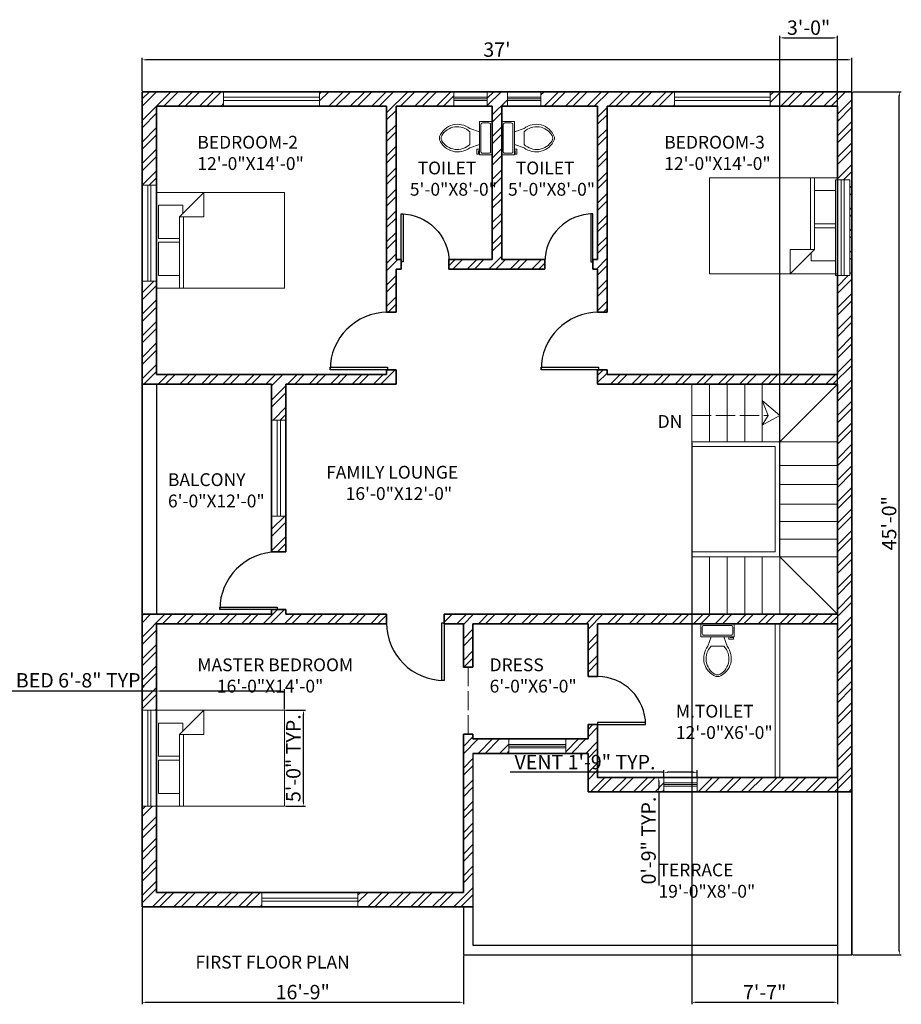
# Model space of a CAD drawing. Units: inches. Extents: x 600 to 1805, y 898 to 2057.
# Tile 5 of 5: x 1172 to 1724, y 1423 to 2039. Entities that reach past the tile are written whole.
import ezdxf

# ---------------------------------------------------------------- set-up
doc = ezdxf.new("R2010")
doc.units = ezdxf.units.IN
doc.linetypes.add('ACAD_ISO02W100', pattern=[15, 12, -3])
for name, color, linetype, lineweight in [('A-ANNO-DIMS', 2, 'Continuous', 18), ('A-ANNO-PATH', 2, 'ACAD_ISO02W100', 13), ('A-ANNO-SYMB', 2, 'Continuous', 13), ('A-ANNO-TEXT', 7, 'Continuous', 25), ('A-AREA-IDEN', 7, 'Continuous', 18), ('A-DOOR', 4, 'Continuous', 25), ('A-DOOR-OVHD', 4, 'ACAD_ISO02W100', 13), ('A-FLOR', 7, 'Continuous', 25), ('A-FLOR-FIXT', 8, 'Continuous', 18), ('A-FLOR-STRS', 3, 'Continuous', 20), ('A-FURN', 8, 'Continuous', 18), ('A-WALL', 7, 'Continuous', 35), ('A-WALL-PATT', 252, 'Continuous', 13)]:
    doc.layers.add(name, color=color, linetype=linetype, lineweight=lineweight)
doc.layers.add('A-GLAZ', color=244, linetype='Continuous', lineweight=20, true_color=0x991b1e)
doc.styles.get("Standard").update_dxf_attribs({"font": 'arial.ttf'})
doc.dimstyles.new('ISO-25', dxfattribs={"dimtxt": 9, "dimasz": 2.5, "dimexe": 1.25, "dimexo": 0.625, "dimtad": 1, "dimlunit": 3, "dimtxsty": 'Standard', "dimcen": 2.5, "dimadec": 0, "dimazin": 0, "dimtfac": 1, "dimtmove": 0, "dimatfit": 3, "dimfxl": 1, "dimarcsym": 0})

# ---------------------------------------------------------------- blocks, each defined once
blk = doc.blocks.new('*D14')
at = {"layer": 'A-ANNO-DIMS', "color": 0, "lineweight": -2, "transparency": 16777216}
for p, q in [((1248.94, 1995), (1248.94, 2015.58)), ((1692.94, 1995), (1692.94, 2015.58)), ((1690.44, 2014.33), (1251.44, 2014.33))]:
    blk.add_line(p, q, dxfattribs=at)
at = {"layer": 'A-ANNO-DIMS', "color": 0, "transparency": 16777216}
for points in [[(1251.44, 2014.74), (1251.44, 2013.91), (1248.94, 2014.33)], [(1690.44, 2014.74), (1690.44, 2013.91), (1692.94, 2014.33)]]:
    blk.add_solid(points, dxfattribs=at)
at = {"layer": 'Defpoints', "color": 0, "transparency": 16777216}
for p in [(1248.94, 2014.33), (1248.94, 1994.38), (1692.94, 1994.38)]:
    blk.add_point(p, dxfattribs=at)
at = {"layer": 'A-ANNO-DIMS', "color": 0, "transparency": 16777216, "insert": (1470.94, 2019.55), "char_height": 9, "attachment_point": 5}
blk.add_mtext("37'", dxfattribs=at)
blk = doc.blocks.new('*U2')
for p, q in [((0, 0), (0, -6)), ((40, 0), (40, -6))]:
    blk.add_line(p, q)
blk.add_lwpolyline([(0, 0), (0, 40), (1.75, 40), (1.75, 0)], close=True)
blk.add_arc((0, 0), 40, 0, 90)
blk = doc.blocks.new('*U5')
for p, q in [((0, 0), (0, 6)), ((40, 0), (40, 6))]:
    blk.add_line(p, q)
blk.add_lwpolyline([(0, 0), (0, -40), (1.75, -40), (1.75, 0)], close=True)
blk.add_arc((0, 0), 40, 270, 0)
blk = doc.blocks.new('*U10')
for p, q in [((9.5, -6), (9.5, -2)), ((-10, -8.5), (-8, -8.5)), ((-10, -9.5), (-10, -8.5)), ((-7, -9.5), (-10, -9.5)), ((-8, -8.5), (-8, -8)), ((-7, -8), (-7, -9.5)), ((-4, -8), (-6, -14)), ((4, -8), (6, -14)), ((4, -14), (-4, -14))]:
    blk.add_line(p, q)
blk.add_lwpolyline([(10.5, -8), (10.5, 0), (-10.5, 0), (-10.5, -8)], close=True)
for points in [[(-9.5, -2), (-9.5, -6)], [(8.5, -1), (-8.5, -1)], [(-8.5, -7), (8.5, -7)]]:
    blk.add_lwpolyline(points)
for centre, radius, start, end in [((-8.62, -1.88), 0.884, 81.8699, 188.1301), ((-8.62, -6.12), 0.884, 171.8699, 278.1301), ((8.62, -1.88), 0.884, 351.8699, 98.1301), ((8.62, -6.12), 0.884, 261.8699, 8.1301), ((3.52, -21.58), 12.17, 141.46911, 247.97143), ((4.2, -21.82), 11.33, 136.36773, 238.94682), ((-3.52, -21.58), 12.17, 292.02843, 38.53071), ((-4.2, -21.82), 11.33, 301.05301, 43.63209), ((0, -27.88), 4, 245.73182, 294.26817), ((0, -29), 4, 254.86053, 285.13947)]:
    blk.add_arc(centre, radius, start, end)
blk = doc.blocks.new('Bed - Queen')
for p, q in [((0, -80.00003), (0, 0)), ((0, 0), (59.99999, 0)), ((59.99999, 0), (59.99999, -80.00003)), ((7.99999, -1.2), (28.79998, -1.2)), ((7.99999, -14.4), (7.99999, -1.2)), ((28.79998, -1.2), (28.79998, -14.4)), ((31.19999, -1.2), (51.99999, -1.2)), ((31.19999, -14.4), (31.19999, -1.2)), ((51.99999, -1.2), (51.99999, -16.4)), ((0, -14.4), (44.8, -14.4)), ((44.8, -16.8), (0, -16.8)), ((59.99999, -29.6), (44.8, -14.4)), ((44.8, -14.4), (44.8, -29.6)), ((51.99999, -16.4), (46.79936, -16.4)), ((44.8, -29.6), (59.99999, -29.6)), ((59.99999, -80.00003), (0, -80.00003))]:
    blk.add_line(p, q)
blk = doc.blocks.new('WIN-60x9')
for p, q in [((60, 5.5), (0, 5.5)), ((60, 3.5), (0, 3.5))]:
    blk.add_line(p, q)
blk.add_lwpolyline([(60, 0), (60, 9), (0, 9), (0, 0)], close=True)
blk = doc.blocks.new('VENT-21x9')
for p, q in [((0, 5.5), (21, 5.5)), ((0, 4.5), (21, 4.5)), ((0, 3.5), (21, 3.5))]:
    blk.add_line(p, q)
blk.add_lwpolyline([(21, 9), (21, 0), (0, 0), (0, 9)], close=True)
blk = doc.blocks.new('*D24')
at = {"layer": 'A-ANNO-DIMS', "color": 0, "lineweight": -2, "transparency": 16777216}
for p, q in [((1575.32, 1568.53), (1479.22, 1568.53)), ((1575.32, 1566), (1575.32, 1569.78)), ((1593.82, 1568.53), (1577.82, 1568.53)), ((1596.32, 1566), (1596.32, 1569.78))]:
    blk.add_line(p, q, dxfattribs=at)
at = {"layer": 'A-ANNO-DIMS', "color": 0, "transparency": 16777216}
for points in [[(1577.82, 1568.94), (1577.82, 1568.11), (1575.32, 1568.53)], [(1593.82, 1568.94), (1593.82, 1568.11), (1596.32, 1568.53)]]:
    blk.add_solid(points, dxfattribs=at)
at = {"layer": 'Defpoints', "color": 0, "transparency": 16777216}
for p in [(1575.32, 1568.53), (1575.32, 1565.38), (1596.32, 1565.38)]:
    blk.add_point(p, dxfattribs=at)
at = {"layer": 'A-ANNO-DIMS', "color": 0, "transparency": 16777216, "insert": (1526.02, 1573.75), "char_height": 9, "attachment_point": 5}
blk.add_mtext('VENT 1\'-9" TYP.', dxfattribs=at)
blk = doc.blocks.new('*D25')
at = {"layer": 'A-ANNO-DIMS', "color": 0, "lineweight": -2, "transparency": 16777216}
for p, q in [((1574.69, 1565.38), (1570.92, 1565.38)), ((1572.17, 1562.88), (1572.17, 1558.88)), ((1574.69, 1556.38), (1570.92, 1556.38)), ((1572.17, 1556.38), (1572.17, 1497.77))]:
    blk.add_line(p, q, dxfattribs=at)
at = {"layer": 'A-ANNO-DIMS', "color": 0, "transparency": 16777216}
for points in [[(1571.75, 1562.88), (1572.58, 1562.88), (1572.17, 1565.38)], [(1571.75, 1558.88), (1572.58, 1558.88), (1572.17, 1556.38)]]:
    blk.add_solid(points, dxfattribs=at)
at = {"layer": 'Defpoints', "color": 0, "transparency": 16777216}
for p in [(1575.32, 1565.38), (1572.17, 1556.38), (1575.32, 1556.38)]:
    blk.add_point(p, dxfattribs=at)
at = {"layer": 'A-ANNO-DIMS', "color": 0, "transparency": 16777216, "insert": (1566.95, 1525.82), "char_height": 9, "attachment_point": 5, "rotation": 90}
blk.add_mtext('0\'-9" TYP.', dxfattribs=at)
blk = doc.blocks.new('*D26')
at = {"layer": 'A-ANNO-DIMS', "color": 0, "lineweight": -2, "transparency": 16777216}
for p, q in [((1257.94, 1608), (1257.94, 1620.63)), ((1337.94, 1608), (1337.94, 1620.63)), ((1257.94, 1619.38), (1121.8, 1619.38)), ((1335.44, 1619.38), (1260.44, 1619.38))]:
    blk.add_line(p, q, dxfattribs=at)
at = {"layer": 'A-ANNO-DIMS', "color": 0, "transparency": 16777216}
for points in [[(1260.44, 1619.79), (1260.44, 1618.96), (1257.94, 1619.38)], [(1335.44, 1619.79), (1335.44, 1618.96), (1337.94, 1619.38)]]:
    blk.add_solid(points, dxfattribs=at)
at = {"layer": 'Defpoints', "color": 0, "transparency": 16777216}
for p in [(1257.94, 1619.38), (1257.94, 1607.38), (1337.94, 1607.38)]:
    blk.add_point(p, dxfattribs=at)
at = {"layer": 'A-ANNO-DIMS', "color": 0, "transparency": 16777216, "insert": (1188.62, 1624.93), "char_height": 9, "attachment_point": 5}
blk.add_mtext('QUEEN BED 6\'-8" TYP.', dxfattribs=at)
blk = doc.blocks.new('*D27')
at = {"layer": 'A-ANNO-DIMS', "color": 0, "lineweight": -2, "transparency": 16777216}
for p, q in [((1338.57, 1607.38), (1351.19, 1607.38)), ((1349.94, 1549.88), (1349.94, 1604.88)), ((1338.57, 1547.38), (1351.19, 1547.38))]:
    blk.add_line(p, q, dxfattribs=at)
at = {"layer": 'A-ANNO-DIMS', "color": 0, "transparency": 16777216}
for points in [[(1349.52, 1604.88), (1350.36, 1604.88), (1349.94, 1607.38)], [(1349.52, 1549.88), (1350.36, 1549.88), (1349.94, 1547.38)]]:
    blk.add_solid(points, dxfattribs=at)
at = {"layer": 'Defpoints', "color": 0, "transparency": 16777216}
for p in [(1337.94, 1607.38), (1349.94, 1607.38), (1337.94, 1547.38)]:
    blk.add_point(p, dxfattribs=at)
at = {"layer": 'A-ANNO-DIMS', "color": 0, "transparency": 16777216, "insert": (1344.72, 1577.38), "char_height": 9, "attachment_point": 5, "rotation": 90}
blk.add_mtext('5\'-0" TYP.', dxfattribs=at)
blk = doc.blocks.new('*D37')
at = {"layer": 'A-ANNO-DIMS', "color": 0, "lineweight": -2, "transparency": 16777216}
for p, q in [((1693.57, 1994.38), (1723.94, 1994.38)), ((1722.69, 1456.88), (1722.69, 1991.88)), ((1693.57, 1454.38), (1723.94, 1454.38))]:
    blk.add_line(p, q, dxfattribs=at)
at = {"layer": 'A-ANNO-DIMS', "color": 0, "transparency": 16777216}
for points in [[(1722.27, 1991.88), (1723.11, 1991.88), (1722.69, 1994.38)], [(1722.27, 1456.88), (1723.11, 1456.88), (1722.69, 1454.38)]]:
    blk.add_solid(points, dxfattribs=at)
at = {"layer": 'Defpoints', "color": 0, "transparency": 16777216}
for p in [(1692.94, 1994.38), (1722.69, 1994.38), (1692.94, 1454.38)]:
    blk.add_point(p, dxfattribs=at)
at = {"layer": 'A-ANNO-DIMS', "color": 0, "transparency": 16777216, "insert": (1717.47, 1724.38), "char_height": 9, "attachment_point": 5, "rotation": 90}
blk.add_mtext('45\'-0"', dxfattribs=at)
blk = doc.blocks.new('*D38')
at = {"layer": 'A-ANNO-DIMS', "color": 0, "lineweight": -2, "transparency": 16777216}
for p, q in [((1248.94, 1483.75), (1248.94, 1423.38)), ((1449.94, 1453.75), (1449.94, 1423.38)), ((1251.44, 1424.63), (1447.44, 1424.63))]:
    blk.add_line(p, q, dxfattribs=at)
at = {"layer": 'A-ANNO-DIMS', "color": 0, "transparency": 16777216}
for points in [[(1251.44, 1425.04), (1251.44, 1424.21), (1248.94, 1424.63)], [(1447.44, 1425.04), (1447.44, 1424.21), (1449.94, 1424.63)]]:
    blk.add_solid(points, dxfattribs=at)
at = {"layer": 'Defpoints', "color": 0, "transparency": 16777216}
for p in [(1248.94, 1484.38), (1449.94, 1454.38), (1449.94, 1424.63)]:
    blk.add_point(p, dxfattribs=at)
at = {"layer": 'A-ANNO-DIMS', "color": 0, "transparency": 16777216, "insert": (1349.44, 1429.85), "char_height": 9, "attachment_point": 5}
blk.add_mtext('16\'-9"', dxfattribs=at)
blk = doc.blocks.new('*D39')
at = {"layer": 'A-ANNO-DIMS', "color": 0, "lineweight": -2, "transparency": 16777216}
for p, q in [((1592.94, 1774.75), (1592.94, 1423.38)), ((1683.94, 1774.75), (1683.94, 1423.38)), ((1595.44, 1424.63), (1681.44, 1424.63))]:
    blk.add_line(p, q, dxfattribs=at)
at = {"layer": 'A-ANNO-DIMS', "color": 0, "transparency": 16777216}
for points in [[(1595.44, 1425.04), (1595.44, 1424.21), (1592.94, 1424.63)], [(1681.44, 1425.04), (1681.44, 1424.21), (1683.94, 1424.63)]]:
    blk.add_solid(points, dxfattribs=at)
at = {"layer": 'Defpoints', "color": 0, "transparency": 16777216}
for p in [(1592.94, 1775.38), (1683.94, 1775.38), (1683.94, 1424.63)]:
    blk.add_point(p, dxfattribs=at)
at = {"layer": 'A-ANNO-DIMS', "color": 0, "transparency": 16777216, "insert": (1638.44, 1429.75), "char_height": 9, "attachment_point": 5}
blk.add_mtext('7\'-7"', dxfattribs=at)
blk = doc.blocks.new('*D40')
at = {"layer": 'A-ANNO-DIMS', "color": 0, "lineweight": -2, "transparency": 16777216}
for p, q in [((1647.94, 1704), (1647.94, 2029.32)), ((1650.44, 2028.07), (1681.44, 2028.07)), ((1683.94, 1704), (1683.94, 2029.32))]:
    blk.add_line(p, q, dxfattribs=at)
at = {"layer": 'A-ANNO-DIMS', "color": 0, "transparency": 16777216}
for points in [[(1650.44, 2028.48), (1650.44, 2027.65), (1647.94, 2028.07)], [(1681.44, 2028.48), (1681.44, 2027.65), (1683.94, 2028.07)]]:
    blk.add_solid(points, dxfattribs=at)
at = {"layer": 'Defpoints', "color": 0, "transparency": 16777216}
for p in [(1683.94, 2028.07), (1647.94, 1703.38), (1683.94, 1703.38)]:
    blk.add_point(p, dxfattribs=at)
at = {"layer": 'A-ANNO-DIMS', "color": 0, "transparency": 16777216, "insert": (1665.94, 2033.29), "char_height": 9, "attachment_point": 5}
blk.add_mtext('3\'-0"', dxfattribs=at)

msp = doc.modelspace()

# ---------------------------------------------------------------- hatches: boundary and pattern name
at = {"layer": 'A-WALL-PATT'}
h = msp.add_hatch(dxfattribs=at)
h.set_pattern_fill('ANSI32', color=256)
h.paths.add_polyline_path([(1581.941, 1994.376), (1498.487, 1994.376), (1498.487, 1985.376), (1533.941, 1985.376), (1533.941, 1889.376), (1530.941, 1889.376), (1530.941, 1887.876), (1530.941, 1883.376), (1533.941, 1883.376), (1533.941, 1856.376), (1539.941, 1856.376), (1539.941, 1985.376), (1581.941, 1985.376)])
h.paths.add_polyline_path([(1443.897, 1994.376), (1359.941, 1994.376), (1359.941, 1985.376), (1401.941, 1985.376), (1401.941, 1856.376), (1407.941, 1856.376), (1407.941, 1883.376), (1410.941, 1883.376), (1410.941, 1887.876), (1410.941, 1889.376), (1407.941, 1889.376), (1407.941, 1985.376), (1443.897, 1985.376)])
h.paths.add_polyline_path([(1299.941, 1994.376), (1248.941, 1994.376), (1248.941, 1935.859), (1257.941, 1935.859), (1257.941, 1985.376), (1299.941, 1985.376)])
h.paths.add_polyline_path([(1257.941, 1875.859), (1248.941, 1875.859), (1248.941, 1811.376), (1329.941, 1811.376), (1329.941, 1788.876), (1338.941, 1788.876), (1338.941, 1811.376), (1407.941, 1811.376), (1407.941, 1820.376), (1401.941, 1820.376), (1401.941, 1817.376), (1257.941, 1817.376)])
h.paths.add_polyline_path([(1338.941, 1728.876), (1329.941, 1728.876), (1329.941, 1706.376), (1338.941, 1706.376)])
h.paths.add_polyline_path([(1401.941, 1667.376), (1338.941, 1667.376), (1338.941, 1670.376), (1333.541, 1670.376), (1329.941, 1670.376), (1329.941, 1667.376), (1248.941, 1667.376), (1248.941, 1607.376), (1257.941, 1607.376), (1257.941, 1661.376), (1401.941, 1661.376)])
h.paths.add_polyline_path([(1323.941, 1493.376), (1257.941, 1493.376), (1257.941, 1547.376), (1248.941, 1547.376), (1248.941, 1484.376), (1323.941, 1484.376)])
h.paths.add_polyline_path([(1500.941, 1889.376), (1473.941, 1889.376), (1473.941, 1985.376), (1477.487, 1985.376), (1477.487, 1994.376), (1464.897, 1994.376), (1464.897, 1985.376), (1467.941, 1985.376), (1467.941, 1889.376), (1440.941, 1889.376), (1440.941, 1883.376), (1500.941, 1883.376)])
h = msp.add_hatch(dxfattribs=at)
h.set_pattern_fill('ANSI32', color=256)
h.paths.add_polyline_path([(1692.941, 1994.376), (1641.941, 1994.376), (1641.941, 1985.376), (1683.941, 1985.376), (1683.941, 1939.293), (1691.741, 1939.293), (1691.741, 1879.293), (1683.941, 1879.293), (1683.941, 1817.376), (1539.941, 1817.376), (1539.941, 1820.376), (1533.941, 1820.376), (1533.941, 1811.376), (1683.941, 1811.376), (1683.941, 1667.376), (1437.941, 1667.376), (1437.941, 1661.376), (1449.941, 1661.376), (1449.941, 1634.376), (1455.941, 1634.376), (1455.941, 1661.376), (1527.941, 1661.376), (1527.941, 1628.376), (1533.941, 1628.376), (1533.941, 1661.376), (1683.941, 1661.376), (1683.941, 1565.376), (1596.318, 1565.376), (1596.318, 1556.376), (1692.941, 1556.376)])
h.paths.add_polyline_path([(1575.318, 1565.376), (1533.941, 1565.376), (1533.941, 1598.376), (1529.441, 1598.376), (1527.941, 1598.376), (1527.941, 1589.376), (1514.038, 1589.376), (1514.038, 1580.376), (1527.941, 1580.376), (1527.941, 1556.376), (1575.318, 1556.376)], flags=17)
h.paths.add_polyline_path([(1478.389, 1589.376), (1455.941, 1589.376), (1455.941, 1592.376), (1449.941, 1592.376), (1449.941, 1493.376), (1383.941, 1493.376), (1383.941, 1484.376), (1455.941, 1484.376), (1455.941, 1580.376), (1478.389, 1580.376)])

# ---------------------------------------------------------------- linework, layer by layer
at = {"layer": 'A-ANNO-PATH'}
msp.add_line((1592.941, 1791.876), (1640.571, 1791.876), dxfattribs=at)
at = {"layer": 'A-ANNO-SYMB'}
for p, q in [((1647.941, 1791.876), (1636.941, 1801.065)), ((1636.941, 1801.065), (1640.571, 1791.876)), ((1640.571, 1791.876), (1636.941, 1785.741)), ((1636.941, 1785.741), (1647.941, 1791.876))]:
    msp.add_line(p, q, dxfattribs=at)
at = {"layer": 'A-DOOR-OVHD'}
msp.add_line((1452.941, 1634.376), (1452.941, 1592.376), dxfattribs=at)
at = {"layer": 'A-FLOR'}
for p, q in [((1257.941, 1811.376), (1257.941, 1667.376)), ((1455.941, 1580.376), (1455.941, 1460.376)), ((1683.941, 1556.376), (1683.941, 1460.376)), ((1449.941, 1484.376), (1449.941, 1454.376)), ((1455.941, 1460.376), (1683.941, 1460.376)), ((1449.941, 1454.376), (1692.941, 1454.376))]:
    msp.add_line(p, q, dxfattribs=at)
at = {"layer": 'A-FLOR-FIXT'}
for p, q in [((1644.941, 1661.376), (1644.941, 1565.376)), ((1647.941, 1661.376), (1647.941, 1565.376))]:
    msp.add_line(p, q, dxfattribs=at)
at = {"layer": 'A-FLOR-STRS'}
for p, q in [((1592.941, 1811.376), (1592.941, 1772.376)), ((1603.941, 1811.376), (1603.941, 1775.376)), ((1614.941, 1811.376), (1614.941, 1775.376)), ((1625.941, 1811.376), (1625.941, 1775.376)), ((1636.941, 1811.376), (1636.941, 1775.376)), ((1647.941, 1811.376), (1647.941, 1667.376)), ((1647.941, 1775.376), (1683.941, 1811.376)), ((1592.941, 1775.376), (1683.941, 1775.376)), ((1592.941, 1772.376), (1644.941, 1772.376)), ((1644.941, 1772.376), (1644.941, 1706.376)), ((1647.941, 1760.409), (1683.941, 1760.409)), ((1647.941, 1748.593), (1683.941, 1748.593)), ((1647.941, 1736.376), (1683.941, 1736.376)), ((1647.941, 1725.376), (1683.941, 1725.376)), ((1647.941, 1714.376), (1683.941, 1714.376)), ((1592.941, 1706.376), (1644.941, 1706.376)), ((1592.941, 1706.376), (1592.941, 1667.376)), ((1592.941, 1703.376), (1683.941, 1703.376)), ((1603.941, 1703.376), (1603.941, 1667.376)), ((1614.941, 1703.376), (1614.941, 1667.376)), ((1625.941, 1703.376), (1625.941, 1667.376)), ((1636.941, 1703.376), (1636.941, 1667.376)), ((1647.941, 1703.376), (1683.941, 1667.376))]:
    msp.add_line(p, q, dxfattribs=at)
at = {"layer": 'A-GLAZ'}
for p, q in [((1478.389, 1585.876), (1514.038, 1585.876)), ((1478.389, 1584.876), (1514.038, 1584.876)), ((1478.389, 1583.876), (1514.038, 1583.876))]:
    msp.add_line(p, q, dxfattribs=at)
msp.add_lwpolyline([(1514.038, 1589.376), (1514.038, 1580.376), (1478.389, 1580.376), (1478.389, 1589.376)], close=True, dxfattribs=at)
at = {"layer": 'A-WALL'}
for p, q in [((1248.941, 1994.376), (1248.941, 1484.376)), ((1248.941, 1994.376), (1692.941, 1994.376)), ((1692.941, 1994.376), (1692.941, 1454.376)), ((1257.941, 1985.376), (1257.941, 1817.376)), ((1257.941, 1985.376), (1401.941, 1985.376)), ((1401.941, 1985.376), (1401.941, 1856.376)), ((1407.941, 1985.376), (1407.941, 1889.376)), ((1407.941, 1985.376), (1467.941, 1985.376)), ((1467.941, 1985.376), (1467.941, 1889.376)), ((1473.941, 1985.376), (1473.941, 1889.376)), ((1473.941, 1985.376), (1533.941, 1985.376)), ((1533.941, 1985.376), (1533.941, 1889.376)), ((1539.941, 1985.376), (1539.941, 1856.376)), ((1539.941, 1985.376), (1683.941, 1985.376)), ((1683.941, 1985.376), (1683.941, 1817.376)), ((1407.941, 1889.376), (1410.941, 1889.376)), ((1410.941, 1889.376), (1410.941, 1883.376)), ((1440.941, 1889.376), (1440.941, 1883.376)), ((1440.941, 1889.376), (1467.941, 1889.376)), ((1473.941, 1889.376), (1500.941, 1889.376)), ((1500.941, 1889.376), (1500.941, 1883.376)), ((1530.941, 1889.376), (1530.941, 1883.376)), ((1530.941, 1889.376), (1533.941, 1889.376)), ((1407.941, 1883.376), (1410.941, 1883.376)), ((1407.941, 1883.376), (1410.941, 1883.376)), ((1407.941, 1883.376), (1407.941, 1856.376)), ((1440.941, 1883.376), (1500.941, 1883.376)), ((1530.941, 1883.376), (1533.941, 1883.376)), ((1533.941, 1883.376), (1533.941, 1856.376)), ((1401.941, 1856.376), (1407.941, 1856.376)), ((1539.941, 1856.376), (1533.941, 1856.376)), ((1257.941, 1817.376), (1401.941, 1817.376)), ((1401.941, 1820.376), (1407.941, 1820.376)), ((1401.941, 1820.376), (1401.941, 1817.376)), ((1407.941, 1820.376), (1407.941, 1811.376)), ((1539.941, 1820.376), (1533.941, 1820.376)), ((1533.941, 1820.376), (1533.941, 1811.376)), ((1539.941, 1820.376), (1539.941, 1817.376)), ((1539.941, 1817.376), (1683.941, 1817.376)), ((1248.941, 1811.376), (1329.941, 1811.376)), ((1329.941, 1811.376), (1329.941, 1706.376)), ((1338.941, 1811.376), (1338.941, 1706.376)), ((1338.941, 1811.376), (1407.941, 1811.376)), ((1533.941, 1811.376), (1683.941, 1811.376)), ((1683.941, 1811.376), (1683.941, 1667.376)), ((1338.941, 1706.376), (1329.941, 1706.376)), ((1338.941, 1670.376), (1329.941, 1670.376)), ((1329.941, 1670.376), (1329.941, 1667.376)), ((1338.941, 1670.376), (1338.941, 1667.376)), ((1248.941, 1667.376), (1329.941, 1667.376)), ((1338.941, 1667.376), (1401.941, 1667.376)), ((1401.941, 1661.376), (1401.941, 1667.376)), ((1437.941, 1661.376), (1437.941, 1667.376)), ((1437.941, 1667.376), (1683.941, 1667.376)), ((1257.941, 1661.376), (1401.941, 1661.376)), ((1257.941, 1661.376), (1257.941, 1493.376)), ((1437.941, 1661.376), (1449.941, 1661.376)), ((1449.941, 1661.376), (1449.941, 1634.376)), ((1455.941, 1661.376), (1455.941, 1634.376)), ((1455.941, 1661.376), (1527.941, 1661.376)), ((1527.941, 1661.376), (1527.941, 1628.376)), ((1533.941, 1661.376), (1533.941, 1628.376)), ((1533.941, 1661.376), (1683.941, 1661.376)), ((1683.941, 1661.376), (1683.941, 1565.376)), ((1455.941, 1634.376), (1449.941, 1634.376)), ((1527.941, 1628.376), (1533.941, 1628.376)), ((1527.941, 1598.376), (1533.941, 1598.376)), ((1527.941, 1598.376), (1527.941, 1589.376)), ((1533.941, 1598.376), (1533.941, 1565.376)), ((1449.941, 1592.376), (1449.941, 1493.376)), ((1455.941, 1592.376), (1449.941, 1592.376)), ((1455.941, 1592.376), (1455.941, 1589.376)), ((1455.941, 1589.376), (1527.941, 1589.376)), ((1455.941, 1580.376), (1527.941, 1580.376)), ((1527.941, 1580.376), (1527.941, 1556.376)), ((1533.941, 1565.376), (1683.941, 1565.376)), ((1527.941, 1556.376), (1692.941, 1556.376)), ((1257.941, 1493.376), (1449.941, 1493.376)), ((1248.941, 1484.376), (1455.941, 1484.376))]:
    msp.add_line(p, q, dxfattribs=at)

# ---------------------------------------------------------------- block references
at = {"layer": 'A-DOOR'}
for name, p, xscale, yscale, zscale, rotation in [('*U5', (1410.941, 1887.876), -0.7499999999999948, 0.7499999999999948, 0.7499999999999948, 180), ('*U5', (1530.941, 1887.876), 0.7499999999999948, 0.7499999999999948, 0.7499999999999948, 180), ('*U2', (1402.541, 1820.376), 0.8999999999999948, 0.8999999999999948, 0.8999999999999948, 89.99999999999999), ('*U2', (1534.541, 1820.376), 0.8999999999999948, 0.8999999999999948, 0.8999999999999948, 89.99999999999999), ('*U2', (1333.541, 1670.376), 0.8999999999999948, 0.8999999999999948, 0.8999999999999948, 89.99999999999999), ('*U2', (1437.941, 1661.976), 0.8999999999999948, 0.8999999999999948, 0.8999999999999948, 180), ('*U5', (1533.941, 1598.376), 0.7499999999999948, 0.7499999999999948, 0.7499999999999948, 89.99999999999999)]:
    msp.add_blockref(name, p, dxfattribs=dict(at, xscale=xscale, yscale=yscale, zscale=zscale, rotation=rotation))
at = {"layer": 'A-FLOR-FIXT', "xscale": -1, "rotation": 270}
msp.add_blockref('*U10', (1467.941, 1965.317), dxfattribs=at)
at = {"layer": 'A-FLOR-FIXT', "rotation": 90}
msp.add_blockref('*U10', (1473.941, 1965.317), dxfattribs=at)
at = {"layer": 'A-FLOR-FIXT', "xscale": -1}
msp.add_blockref('*U10', (1608.941, 1661.376), dxfattribs=at)
at = {"layer": 'A-FURN'}
for p, rotation in [((1683.941, 1940.493), 270), ((1257.941, 1871.376), 90), ((1257.941, 1547.376), 90)]:
    msp.add_blockref('Bed - Queen', p, dxfattribs=dict(at, rotation=rotation))
at = {"layer": 'A-GLAZ'}
for name, p in [('WIN-60x9', (1299.941, 1985.376)), ('VENT-21x9', (1443.896, 1985.376)), ('VENT-21x9', (1477.487, 1985.376)), ('WIN-60x9', (1581.941, 1985.376)), ('WIN-60x9', (1323.941, 1484.376))]:
    msp.add_blockref(name, p, dxfattribs=at)
for name, p, rotation in [('WIN-60x9', (1257.941, 1875.859), 90.00000000000067), ('WIN-60x9', (1691.741, 1879.293), 90.00000000000153), ('WIN-60x9', (1338.941, 1728.876), 90.00000000000183), ('WIN-60x9', (1257.941, 1547.376), 90.00000000000081), ('VENT-21x9', (1596.318, 1565.376), 180)]:
    msp.add_blockref(name, p, dxfattribs=dict(at, rotation=rotation))

# ---------------------------------------------------------------- texts
at = {"layer": 'A-ANNO-TEXT', "char_height": 8, "attachment_point": 1}
for s, width, insert in [('DN', 17.03025, (1571.516, 1792.048)), ('FIRST FLOOR PLAN', 107.5421, (1282.294, 1453.756))]:
    msp.add_mtext_dynamic_manual_height_columns(s, width=width, gutter_width=12.5, heights=[0], dxfattribs=dict(at, insert=insert))
at = {"layer": 'A-AREA-IDEN', "char_height": 8, "attachment_point": 1}
for s, width, insert in [('BEDROOM-2\\P12\'-0"X14\'-0"', 75.22987, (1283.53, 1966.753)), ('BEDROOM-3\\P12\'-0"X14\'-0"', 75.22987, (1575.623, 1966.753)), ('  TOILET\\P5\'-0"X8\'-0"', 51.4853, (1416.456, 1950.642)), ('  TOILET\\P5\'-0"X8\'-0"', 51.4853, (1477.861, 1950.642)), ('BALCONY\\P6\'-0"X12\'-0"', 59.62904, (1265.109, 1755.632)), ('FAMILY LOUNGE\\P     16\'-0"X12\'-0"', 107.24342, (1364.095, 1760.267)), ('MASTER BEDROOM\\P     16\'-0"X14\'-0"', 107.24342, (1283.53, 1639.779)), ('DRESS\\P6\'-0"X6\'-0"', 57.73206, (1466.356, 1639.779)), ('M.TOILET\\P12\'-0"X6\'-0"', 57.73206, (1582.92, 1610.754)), ('TERRACE\\P19\'-0"X8\'-0"', 58.24382, (1572.043, 1511.432))]:
    msp.add_mtext_dynamic_manual_height_columns(s, width=width, gutter_width=12.5, heights=[0], dxfattribs=dict(at, insert=insert))

# ---------------------------------------------------------------- dimensions: what is measured, and where the dimension line sits
at = {"layer": 'A-ANNO-DIMS'}
for base, p1, p2, override, picture, middle in [((1683.941, 2028.067), (1647.941, 1703.376), (1683.941, 1703.376), {"dimdec": 1, "dimlfac": 1, "dimrnd": 0, "dimzin": 1, "dimdsep": 46, "dimlunit": 4, "dimfrac": 2}, '*D40', (1665.941, 2033.291)), ((1248.941, 2014.328), (1692.941, 1994.376), (1248.941, 1994.376), {"dimclrd": 0, "dimclre": 0, "dimclrt": 0}, '*D14', (1470.941, 2019.552)), ((1683.941, 1424.626), (1592.941, 1775.376), (1683.941, 1775.376), {"dimdec": 1, "dimlfac": 1, "dimrnd": 0, "dimzin": 1, "dimdsep": 46, "dimlunit": 4, "dimfrac": 2}, '*D39', (1638.441, 1429.751)), ((1449.941, 1424.626), (1248.941, 1484.376), (1449.941, 1454.376), {"dimdec": 1, "dimlfac": 1, "dimrnd": 0, "dimzin": 1, "dimdsep": 46, "dimlunit": 4, "dimfrac": 2}, '*D38', (1349.441, 1429.846))]:
    dim = msp.add_linear_dim(base=base, p1=p1, p2=p2, dimstyle='ISO-25', override=override, dxfattribs=at)
    dim.commit()
    dim.dimension.update_dxf_attribs({"geometry": picture, "text_midpoint": middle})
dim = msp.add_linear_dim(base=(1722.691, 1994.376), p1=(1692.941, 1454.376), p2=(1692.941, 1994.376), angle=90, dimstyle='ISO-25', override={"dimdec": 1, "dimlfac": 1, "dimrnd": 0, "dimzin": 1, "dimdsep": 46, "dimlunit": 4, "dimfrac": 2}, dxfattribs=at)
dim.commit()
dim.dimension.update_dxf_attribs({"geometry": '*D37', "text_midpoint": (1717.471, 1724.376)})
for base, p1, p2, angle, text, picture, middle in [((1257.941, 1619.376), (1337.941, 1607.376), (1257.941, 1607.376), 180, 'QUEEN BED <> TYP.', '*D26', (1188.621, 1624.931)), ((1349.941, 1607.376), (1337.941, 1547.376), (1337.941, 1607.376), 90, '<> TYP.', '*D27', (1344.721, 1577.376)), ((1575.318, 1568.526), (1596.318, 1565.376), (1575.318, 1565.376), 180, 'VENT <> TYP.', '*D24', (1526.017, 1573.746)), ((1572.168, 1556.376), (1575.318, 1565.376), (1575.318, 1556.376), 270, '<> TYP.', '*D25', (1566.948, 1525.821))]:
    dim = msp.add_linear_dim(base=base, p1=p1, p2=p2, angle=angle, text=text, dimstyle='ISO-25', override={"dimdec": 1, "dimlfac": 1, "dimrnd": 0, "dimzin": 1, "dimdsep": 46, "dimlunit": 4, "dimfrac": 2}, dxfattribs=at)
    dim.commit()
    dim.dimension.update_dxf_attribs({"geometry": picture, "text_midpoint": middle})

doc.saveas('drawing.dxf')
